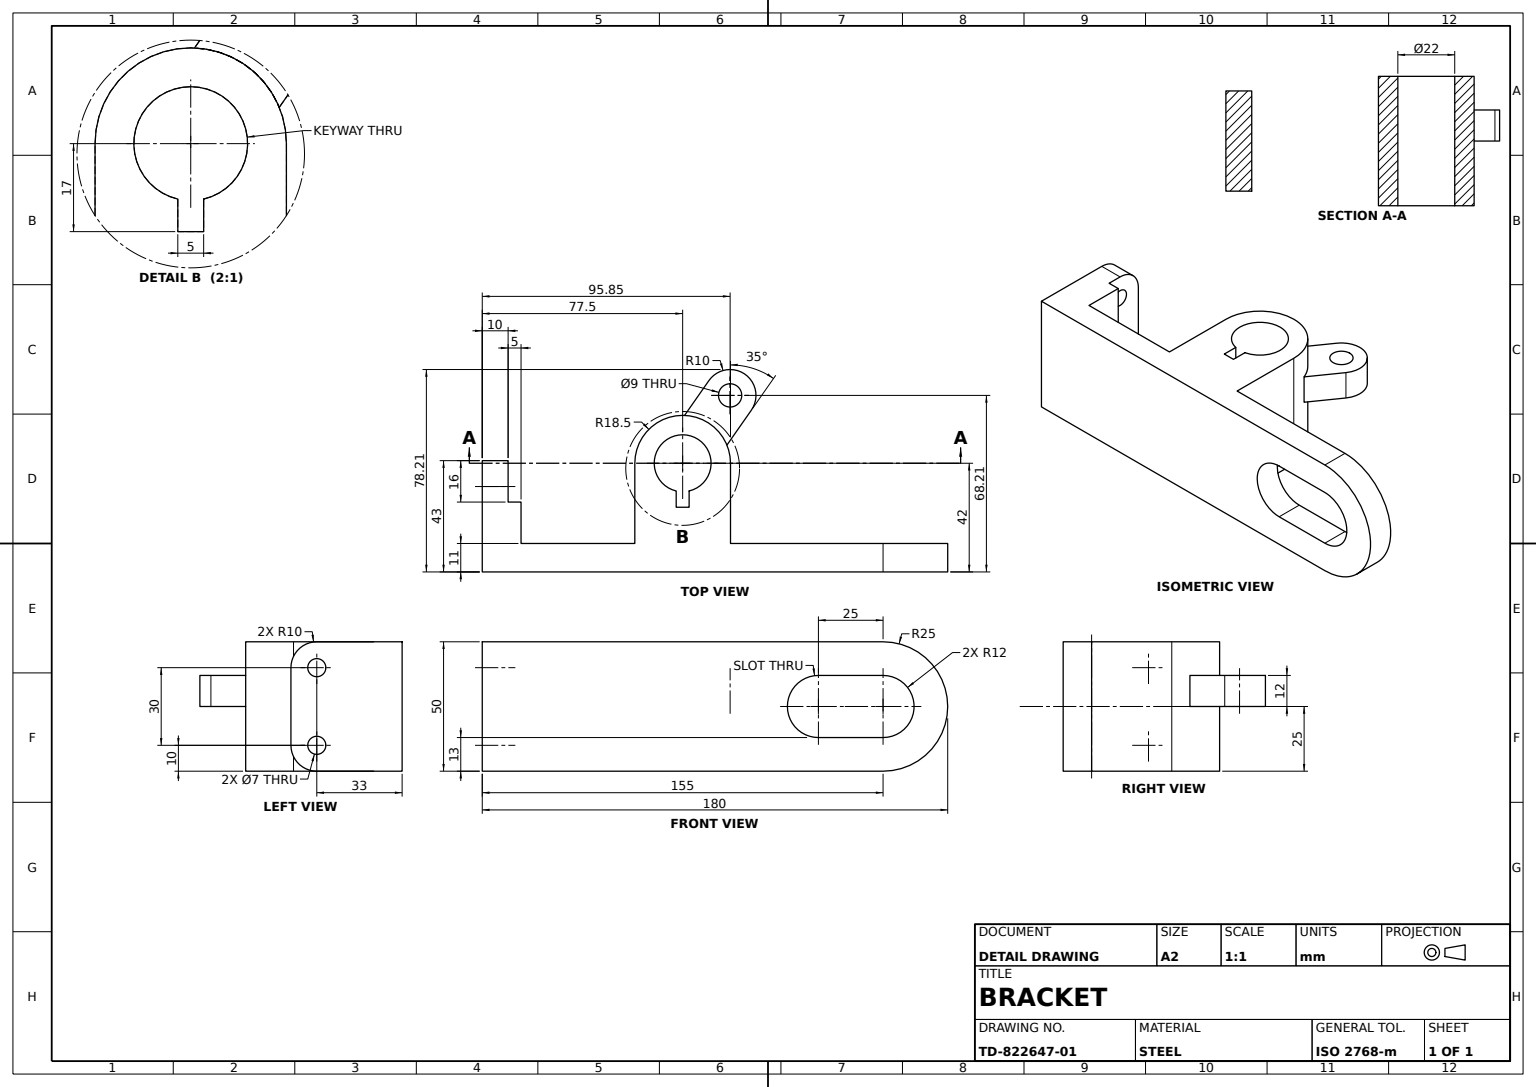
from build123d import *

# Parameters (mm, degrees)
SLOTTED_ARM_PLATE_DEPTH   = 11
END_WALL_DEPTH            = 25
END_WALL_FILLET_R10_R     = 10
WALL_NOTCH_SKETCH_R       = 3.5
WALL_NOTCH_CUT_DEPTH      = 25
HUB_WITH_KEYED_BORE_DEPTH = 25
EYE_START                 = 12
EYE_LUG_SKETCH_R          = 4.5
EYE_LUG_DEPTH             = 12


with BuildPart() as part:
    # Slotted Arm Sketch → Slotted Arm Plate (new body)
    with BuildSketch(Plane.XY):
        with BuildLine():
            Line((-77.5, 25), (77.5, 25))
            ThreePointArc((77.5, 25), (102.5, 0), (77.5, -25))
            Line((77.5, -25), (-77.5, -25))
            Line((-77.5, -25), (-77.5, 25))
        make_face()
        with BuildLine():
            Line((52.5, 12), (77.5, 12))
            ThreePointArc((77.5, 12), (89.5, 0), (77.5, -12))
            Line((77.5, -12), (52.5, -12))
            ThreePointArc((52.5, -12), (40.5, 0), (52.5, 12))
        make_face(mode=Mode.SUBTRACT)
    extrude(amount=SLOTTED_ARM_PLATE_DEPTH)

    # End Wall Sketch → End Wall (add, symmetric)
    with BuildSketch(Plane(origin=(0, 0, 0), x_dir=(1, 0, 0), z_dir=(0, 1, 0))):
        Polygon((-77.5, 0), (-77.5, 32), (-67.5, 32), (-67.5, 16), (-62.5, 16), (-62.5, 0), align=None)
    extrude(amount=END_WALL_DEPTH, both=True)

    # End Wall Fillet R10
    end_wall_fillet_r10_edges = [part.edges().sort_by_distance(p)[0] for p in [
        (-72.5, -25, -32),
        (-72.5, 25, -32),
    ]]
    fillet(end_wall_fillet_r10_edges, radius=END_WALL_FILLET_R10_R)

    # Wall Notch Sketch → Wall Notch Cut (cut, symmetric)
    with BuildSketch(Plane.ZY.offset(77.5)):
        with Locations((-22, 15)):
            Circle(WALL_NOTCH_SKETCH_R)
        with Locations((-22, -15)):
            Circle(WALL_NOTCH_SKETCH_R)
    extrude(amount=WALL_NOTCH_CUT_DEPTH, both=True, mode=Mode.SUBTRACT)

    # Hub Sketch → Hub With Keyed Bore (add, symmetric)
    with BuildSketch(Plane(origin=(0, 0, 0), x_dir=(1, 0, 0), z_dir=(0, 1, 0))):
        with BuildLine():
            Line((18.5, 0), (18.5, 31))
            ThreePointArc((18.5, 31), (0, 49.5), (-18.5, 31))
            Line((-18.5, 31), (-18.5, 0))
            Line((-18.5, 0), (18.5, 0))
        make_face()
        with BuildLine():
            ThreePointArc((2.5, 20.287857357), (0, 42), (-2.5, 20.287857357))
            Line((-2.5, 20.287857357), (-2.5, 14))
            Line((-2.5, 14), (2.5, 14))
            Line((2.5, 14), (2.5, 20.287857357))
        make_face(mode=Mode.SUBTRACT)
    extrude(amount=HUB_WITH_KEYED_BORE_DEPTH, both=True)

    # Eye Lug Sketch → Eye Lug (add)
    with BuildSketch(Plane(origin=(0, 0, 0), x_dir=(1, 0, 0), z_dir=(0, 1, 0)).offset(EYE_START)):
        with BuildLine():
            Line((17.118883443, 38.013831311), (26.545966406, 51.477101054))
            ThreePointArc((26.545966406, 51.477101054), (24.090210327, 65.40438586), (10.16292552, 62.948629781))
            Line((10.16292552, 62.948629781), (0.735842557, 49.485360038))
            ThreePointArc((0.735842557, 49.485360038), (10.611164072, 46.154312819), (17.118883443, 38.013831311))
        make_face()
        with Locations(Location((18.354445963, 57.212865417, 0), (0, 0, 270))):
            Circle(EYE_LUG_SKETCH_R, mode=Mode.SUBTRACT)
    extrude(amount=-EYE_LUG_DEPTH)


solid = part.part
